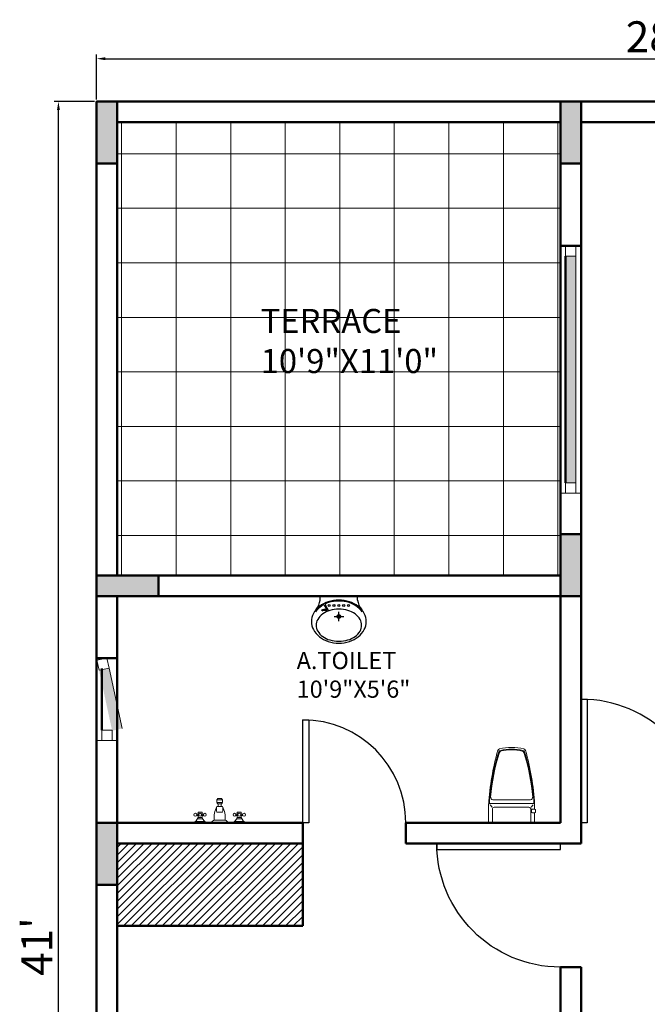
# Model space of a CAD drawing. Units: inches. Extents: x 3064 to 19385, y 846 to 15425.
# Tile 18 of 108: x 3625 to 3808, y 1134 to 1420. Entities that reach past the tile are written whole.
import ezdxf

# ---------------------------------------------------------------- set-up
doc = ezdxf.new("R2010")
doc.units = ezdxf.units.IN
for name, color, linetype, lineweight in [('A-ANNO-DIMS', 2, 'Continuous', 18), ('A-AREA-IDEN', 3, 'Continuous', 18), ('A-COLS', 1, 'Continuous', 35), ('A-DOOR', 3, 'Continuous', 25), ('A-FLOR-FIXT', 9, 'Continuous', 18), ('A-FLOR-PATT', 252, 'Continuous', 13), ('A-FURN-PATT', 252, 'Continuous', 13), ('A-GLAZ', 4, 'Continuous', 18), ('A-WALL', 7, 'Continuous', 50)]:
    doc.layers.add(name, color=color, linetype=linetype, lineweight=lineweight)
doc.layers.add('THIET-BI', color=21, linetype='Continuous')
doc.styles.get("Standard").update_dxf_attribs({"font": 'arial.ttf'})
doc.dimstyles.new('ISO-25', dxfattribs={"dimtxt": 9, "dimasz": 2.5, "dimexe": 1.25, "dimexo": 0.625, "dimtad": 1, "dimdec": 1, "dimlunit": 3, "dimtxsty": 'Standard', "dimcen": 2.5, "dimadec": 0, "dimazin": 0, "dimtfac": 1, "dimtdec": 1, "dimtmove": 0, "dimatfit": 3, "dimfxl": 1, "dimarcsym": 0})

# ---------------------------------------------------------------- blocks, each defined once
blk = doc.blocks.new('*U3')
for p, q in [((0, 0), (0, -6)), ((36, 0), (36, -6))]:
    blk.add_line(p, q)
blk.add_lwpolyline([(0, 0), (0, 36), (1.75, 36), (1.75, 0)], close=True)
blk.add_arc((0, 0), 36, 0, 90)
blk = doc.blocks.new('*U4')
for p, q in [((0, 0), (0, -6)), ((30, 0), (30, -6))]:
    blk.add_line(p, q)
blk.add_lwpolyline([(0, 0), (0, 30), (1.75, 30), (1.75, 0)], close=True)
blk.add_arc((0, 0), 30, 0, 90)
blk = doc.blocks.new('A$C430D11A0')
at = {"layer": 'THIET-BI'}
for p, q in [((90, 445), (90, 485)), ((475, 485), (90, 485)), ((475, 483), (90, 483)), ((475, 445), (475, 485)), ((129, 398), (158, 344)), ((138, 403), (176, 332)), ((282, 226), (282, 325)), ((233, 275), (332, 275))]:
    blk.add_line(p, q, dxfattribs=at)
for points in [[(565, 223, 0.121635), (545, 305, 0.10526), (482, 380, 0.088175), (393, 427, 0.079002), (282, 445, 0.079002), (172, 427, 0.088175), (83, 380, 0.10526), (20, 305, 0.121635), (0, 223, 0.121635), (20, 140, 0.10526), (83, 65, 0.088175), (172, 18, 0.079002), (282, 0, 0.079002), (393, 18, 0.088175), (482, 65, 0.10526), (545, 140, 0.121635)], [(517, 185, 0.134042), (501, 245, 0.106817), (449, 302, 0.082468), (376, 337, 0.070874), (282, 350, 0.070874), (189, 337, 0.082468), (116, 302, 0.106817), (64, 245, 0.134042), (47, 185, 0.134042), (64, 125, 0.106817), (116, 68, 0.082468), (189, 33, 0.070874), (282, 20, 0.070874), (376, 33, 0.082468), (449, 68, 0.106817), (501, 125, 0.134042)]]:
    blk.add_lwpolyline(points, format="xyb", close=True, dxfattribs=at)
for points in [[(523, 322, 0.07708), (476, 372, 0.088175), (390, 418, 0.079002), (282, 435, 0.079002), (175, 418, 0.035427), (138, 403, 0.07708)], [(129, 398, 0.043566), (89, 372, 0.07708), (42, 322, 0.041486)]]:
    blk.add_lwpolyline(points, format="xyb", dxfattribs=at)
for centre, radius in [((182, 388), 10.5), ((232, 388), 10.5), ((282, 388), 10.5), ((332, 388), 10.5), ((382, 388), 10.5), ((282, 275), 20), ((282, 275), 15)]:
    blk.add_circle(centre, radius, dxfattribs=at)
for centre, radius, start, end in [((-104, 469), 195, 320.8253, 352.9557), ((669, 469), 195, 187.0443, 219.1747), ((136, 285), 62.9, 69.643, 123.4774), ((136, 285), 52.9, 55.2455, 123.4774)]:
    blk.add_arc(centre, radius, start, end, dxfattribs=at)
blk = doc.blocks.new('WC-P05')
for p, q in [((-202, 532), (-202, 439)), ((-192, 542), (263, 542)), ((-163, 542), (-163, 401)), ((234, 542), (234, 401)), ((273, 532), (273, 352)), ((-210, 430), (-210, 409)), ((-201, 439), (-180, 439)), ((-171, 430), (-171, 409)), ((-202, 400), (-202, 352)), ((-201, 400), (-180, 400)), ((-192, 342), (263, 342)), ((-167, 379), (-188, 357)), ((-143, 381), (214, 381)), ((237, 379), (258, 357)), ((-159, 303), (229, 303))]:
    blk.add_line(p, q)
blk.add_lwpolyline([(-91, -222, 0.114547), (161, -222, 0.114547)], format="xyb")
for centre, radius, start, end in [((-192, 532), 10, 90, 180), ((263, 532), 10, 0, 90), ((-201, 430), 9, 90, 180), ((-201, 409), 9, 180, 270), ((-180, 430), 9, 0, 90), ((-180, 409), 9, 270, 0), ((2309, 492), 2515, 183.2067, 196.1242), ((-192, 352), 10, 180, 270), ((1906, 447), 2103, 182.8743, 197.6554), ((-143, 401), 20, 180, 270), ((-1836, 447), 2103, 342.3446, 357.1257), ((-2239, 492), 2515, 343.8727, 356.7933), ((214, 401), 20, 270, 0), ((263, 352), 10, 270, 0), ((-159, 280), 22.5, 90, 184.6246), ((1906, 447), 2095, 184.6245, 197.5277), ((-1836, 447), 2095, 342.464, 355.3754), ((229, 280), 22.5, 355.3754, 90), ((-76, -184), 22.5, 197.6554, 257.5059), ((-70, -177), 22.5, 197.5277, 258.1005), ((36, 324), 535, 258.1005, 281.7373), ((140, -177), 22.5, 281.7373, 342.464), ((146, -184), 22.5, 282.4941, 342.3446), ((-86, -200), 22.5, 196.1242, 256.8994), ((35, 318), 536, 257.5059, 282.4941), ((156, -200), 22.5, 283.0378, 343.8727)]:
    blk.add_arc(centre, radius, start, end)
blk = doc.blocks.new('Faucet - Bathroom front')
for p, q in [((-0.5, 4.25), (0.5, 4.25)), ((0.5, 3.75), (-0.5, 3.75)), ((-0.5, 3), (0.5, 3)), ((0.5, 2), (-0.5, 2)), ((-0.25, 3), (-0.25, 3.5)), ((0.25, 3.5), (0.25, 3)), ((-5, 0), (-2.25, 0)), ((-4.5087, 0.25), (-2.7408, 0.25)), ((-4, 1.625), (-4.25, 1.625)), ((-4, 1.375), (-4.25, 1.375)), ((-3.1442, 0.75), (-4.0979, 0.75)), ((-3.25, 1.625), (-3, 1.625)), ((-3.25, 1.375), (-3, 1.375)), ((-1.5, 0), (1.5, 0)), ((-1, 0.5), (1, 0.5)), ((2.25, 0), (5, 0)), ((2.7413, 0.25), (4.5092, 0.25)), ((3.25, 1.625), (3, 1.625)), ((3.25, 1.375), (3, 1.375)), ((4.1058, 0.75), (3.1521, 0.75)), ((4, 1.625), (4.25, 1.625)), ((4, 1.375), (4.25, 1.375))]:
    blk.add_line(p, q)
for points in [[(-0.5, 3.75), (-0.5, 4.25)], [(-0.25, 4.5), (0.25, 4.5)], [(0.5, 4.25), (0.5, 3.75)], [(0.25, 3.5), (-0.25, 3.5)]]:
    blk.add_lwpolyline(points)
for points in [[(-4, 1), (-4, 2), (-3.25, 2), (-3.25, 1)], [(3.25, 1), (3.25, 2), (4, 2), (4, 1)]]:
    blk.add_lwpolyline(points, close=True)
for centre in [(-4.5, 1.5), (-3.625, 1.5), (-2.75, 1.5), (2.75, 1.5), (3.625, 1.5), (4.5, 1.5)]:
    blk.add_circle(centre, 0.2795)
for centre, radius, start, end in [((-0.2575, 4.2575), 0.2426, 88.22243, 181.7776), ((-0.2575, 3.7425), 0.2426, 178.2224, 271.7776), ((0.2575, 4.2575), 0.2426, 358.2224, 91.77757), ((0.2575, 3.7425), 0.2426, 268.2224, 1.777565), ((3, 1), 4.0311, 150.2551, 187.125), ((0.6413, 2.5), 1.246, 156.3417, 203.6583), ((-3, 1), 4.0311, 352.875, 29.74488), ((-0.6413, 2.5), 1.246, 336.3417, 23.65835), ((-5.375, 1.375), 1.4252, 285.2551, 344.7449), ((-1.875, 1.375), 1.4252, 195.2551, 254.7449), ((-0.7962, -0.2038), 0.7327, 106.1502, 163.8498), ((0.7962, -0.2038), 0.7327, 16.1502, 73.84979), ((1.875, 1.375), 1.4252, 285.2551, 344.7449), ((5.375, 1.375), 1.4252, 195.2551, 254.7449)]:
    blk.add_arc(centre, radius, start, end)
blk = doc.blocks.new('*D40')
at = {"layer": 'A-ANNO-DIMS', "color": 0, "lineweight": -2, "transparency": 16777216}
for p, q in [((3646.73, 1396.34), (3634.99, 1396.34)), ((3636.24, 906.84), (3636.24, 1393.84)), ((3646.73, 904.34), (3634.99, 904.34))]:
    blk.add_line(p, q, dxfattribs=at)
at = {"layer": 'A-ANNO-DIMS', "color": 0, "transparency": 16777216}
for points in [[(3635.82, 1393.84), (3636.66, 1393.84), (3636.24, 1396.34)], [(3635.82, 906.84), (3636.66, 906.84), (3636.24, 904.34)]]:
    blk.add_solid(points, dxfattribs=at)
at = {"layer": 'Defpoints', "color": 0, "transparency": 16777216}
for p in [(3636.24, 1396.34), (3647.36, 1396.34), (3647.36, 904.34)]:
    blk.add_point(p, dxfattribs=at)
at = {"layer": 'A-ANNO-DIMS', "color": 0, "transparency": 16777216, "insert": (3631.1, 1150.34), "char_height": 9, "attachment_point": 5, "rotation": 90}
blk.add_mtext("41'", dxfattribs=at)
blk = doc.blocks.new('*D41')
at = {"layer": 'A-ANNO-DIMS', "color": 0, "lineweight": -2, "transparency": 16777216}
for p, q in [((3647.36, 1396.96), (3647.36, 1410.06)), ((3649.86, 1408.81), (3986.86, 1408.81)), ((3989.36, 1396.96), (3989.36, 1410.06))]:
    blk.add_line(p, q, dxfattribs=at)
at = {"layer": 'A-ANNO-DIMS', "color": 0, "transparency": 16777216}
for points in [[(3649.86, 1409.23), (3649.86, 1408.39), (3647.36, 1408.81)], [(3986.86, 1409.23), (3986.86, 1408.39), (3989.36, 1408.81)]]:
    blk.add_solid(points, dxfattribs=at)
at = {"layer": 'Defpoints', "color": 0, "transparency": 16777216}
for p in [(3989.36, 1408.81), (3647.36, 1396.34), (3989.36, 1396.34)]:
    blk.add_point(p, dxfattribs=at)
at = {"layer": 'A-ANNO-DIMS', "color": 0, "transparency": 16777216, "insert": (3818.36, 1414.03), "char_height": 9, "attachment_point": 5}
blk.add_mtext('28\'-6"', dxfattribs=at)
blk = doc.blocks.new('WIN-600')
h = blk.add_hatch(color=256)
h.dxf.hatch_style = 1
h.paths.add_polyline_path([(3, 18), (0, 18), (0, 0), (3, 0)])
blk.add_line((3, 18), (3, 0))
blk.add_lwpolyline([(3, 18), (0, 18), (0, 21), (3, 21)], close=True)
blk = doc.blocks.new('WIN-1900')
blk.add_line((3, 0), (3, 66))
blk.add_lwpolyline([(3, 66), (0, 66), (0, 69), (3, 69)], close=True)

msp = doc.modelspace()

# ---------------------------------------------------------------- hatches: boundary and pattern name
at = {"layer": 'A-COLS'}
h = msp.add_hatch(color=256, dxfattribs=at)
h.dxf.hatch_style = 1
h.paths.add_polyline_path([(3647.36, 1378.34), (3653.36, 1378.34), (3653.36, 1396.34), (3647.36, 1396.34)])
h = msp.add_hatch(color=256, dxfattribs=at)
h.dxf.hatch_style = 1
h.paths.add_polyline_path([(3782.36, 1378.34), (3788.36, 1378.34), (3788.36, 1396.34), (3782.36, 1396.34)])
h = msp.add_hatch(color=256, dxfattribs=at)
h.dxf.hatch_style = 1
h.paths.add_polyline_path([(3782.36, 1252.34), (3788.36, 1252.34), (3788.36, 1270.34), (3782.36, 1270.34)])
h = msp.add_hatch(color=256, dxfattribs=at)
h.dxf.hatch_style = 1
h.paths.add_polyline_path([(3665.36, 1252.34), (3665.36, 1258.34), (3647.36, 1258.34), (3647.36, 1252.34)])
h = msp.add_hatch(color=256, dxfattribs=at)
h.dxf.hatch_style = 1
h.paths.add_polyline_path([(3647.36, 1168.34), (3653.36, 1168.34), (3653.36, 1186.34), (3647.36, 1186.34)])
at = {"layer": 'A-FLOR-PATT'}
h = msp.add_hatch(dxfattribs=at)
h.set_pattern_fill('ANSI37', color=256, scale=5, angle=45)
h.set_pattern_definition([(90, (-695.134, 0), (-15.875, 0), []), (180, (-695.134, 0), (-2e-15, -15.875), [])])
h.paths.add_polyline_path([(3653.36, 1390.34), (3653.36, 1378.34), (3653.36, 1258.34), (3782.36, 1258.34), (3782.36, 1270.34), (3782.36, 1390.34)])
at = {"layer": 'A-FURN-PATT'}
h = msp.add_hatch(dxfattribs=at)
h.set_pattern_fill('ANSI31', color=256, scale=0.5)
h.set_pattern_definition([(45, (-695.1336, -6), (-1.122532, 1.122532), [])])
h.paths.add_polyline_path([(3707.36, 1180.34), (3653.36, 1180.34), (3653.36, 1162.34), (3653.36, 1156.34), (3707.36, 1156.34)])
at = {"layer": 'A-GLAZ'}
h = msp.add_hatch(color=256, dxfattribs=at)
h.dxf.hatch_style = 1
h.paths.add_polyline_path([(3783.86, 1285.34), (3786.86, 1285.34), (3786.86, 1351.34), (3783.86, 1351.34)])

# ---------------------------------------------------------------- linework, layer by layer
for p, q in [((3788.36, 1282.34), (3782.36, 1282.34)), ((3647.36, 1210.28), (3653.36, 1210.28))]:
    msp.add_line(p, q, dxfattribs=at)
for points in [[(3786.86, 1282.34), (3783.86, 1282.34), (3783.86, 1285.34), (3786.86, 1285.34)], [(3651.86, 1210.28), (3648.86, 1210.28), (3648.86, 1213.28), (3651.86, 1213.28)]]:
    msp.add_lwpolyline(points, close=True, dxfattribs=at)
at = {"layer": 'A-WALL'}
for p, q in [((3989.36, 1396.34), (3647.36, 1396.34)), ((3647.36, 1396.34), (3647.36, 976.34)), ((3782.36, 1390.34), (3653.36, 1390.34)), ((3653.36, 1390.34), (3653.36, 1258.34)), ((3782.36, 1390.34), (3782.36, 1258.34)), ((3983.36, 1390.34), (3788.36, 1390.34)), ((3788.36, 1390.34), (3788.36, 1180.34)), ((3782.36, 1354.34), (3788.36, 1354.34)), ((3783.86, 1351.34), (3783.86, 1285.34)), ((3653.36, 1258.34), (3782.36, 1258.34)), ((3653.36, 1252.34), (3782.36, 1252.34)), ((3653.36, 1252.34), (3653.36, 1186.34)), ((3788.36, 1252.34), (3782.36, 1252.34)), ((3782.36, 1252.34), (3782.36, 1186.34)), ((3647.36, 1234.28), (3653.36, 1234.28)), ((3648.86, 1231.28), (3648.86, 1213.28)), ((3653.36, 1186.34), (3707.36, 1186.34)), ((3707.36, 1186.34), (3707.36, 1156.34)), ((3737.36, 1186.34), (3737.36, 1180.34)), ((3737.36, 1186.34), (3782.36, 1186.34)), ((3653.36, 1180.34), (3707.36, 1180.34)), ((3653.36, 1180.34), (3653.36, 982.34)), ((3737.36, 1180.34), (3788.36, 1180.34)), ((3653.36, 1156.34), (3707.36, 1156.34)), ((3782.36, 1144.34), (3788.36, 1144.34)), ((3782.36, 1144.34), (3782.36, 982.34)), ((3788.36, 1144.34), (3788.36, 976.34))]:
    msp.add_line(p, q, dxfattribs=at)
for points in [[(3653.36, 1378.34), (3653.36, 1396.34), (3647.36, 1396.34), (3647.36, 1378.34)], [(3788.36, 1378.34), (3788.36, 1396.34), (3782.36, 1396.34), (3782.36, 1378.34)], [(3788.36, 1252.34), (3788.36, 1270.34), (3782.36, 1270.34), (3782.36, 1252.34)], [(3665.36, 1258.34), (3647.36, 1258.34), (3647.36, 1252.34), (3665.36, 1252.34)], [(3653.36, 1168.34), (3653.36, 1186.34), (3647.36, 1186.34), (3647.36, 1168.34)]]:
    msp.add_lwpolyline(points, close=True, dxfattribs=at)

# ---------------------------------------------------------------- block references
at = {"layer": 'A-DOOR'}
for name, p in [('*U3', (3788.36, 1186.34)), ('*U4', (3707.36, 1186.34))]:
    msp.add_blockref(name, p, dxfattribs=at)
at = {"layer": 'A-DOOR', "xscale": -1, "rotation": 90}
msp.add_blockref('*U3', (3782.36, 1180.34), dxfattribs=at)
at = {"layer": 'A-FLOR-FIXT'}
for name, p, xscale, yscale, zscale in [('A$C430D11A0', (3709.89, 1238.65), 0.0282220760332506, 0.0282220760332506, 0.0282220760332506), ('Faucet - Bathroom front', (3683.17, 1186.34), 1.573166238287219, 1.573166238287219, 1.573166238287219)]:
    msp.add_blockref(name, p, dxfattribs=dict(at, xscale=xscale, yscale=yscale, zscale=zscale))
at = {"layer": 'A-FLOR-FIXT', "xscale": 0.0282220760332506, "yscale": 0.0282220760332506, "zscale": 0.0282220760332506, "rotation": 180}
msp.add_blockref('WC-P05', (3769.14, 1201.63), dxfattribs=at)
at = {"layer": 'A-GLAZ'}
msp.add_blockref('WIN-1900', (3783.86, 1285.34), dxfattribs=at)
at = {"layer": 'A-GLAZ', "rotation": 12.21571913412907}
msp.add_blockref('WIN-600', (3651.87, 1213.17), dxfattribs=at)

# ---------------------------------------------------------------- texts
at = {"layer": 'A-AREA-IDEN', "attachment_point": 1}
for s, insert, char_height in [('TERRACE\\P10\'9"X11\'0"', (3695.09, 1335.96), 7), ('A.TOILET\\P10\'9"X5\'6"', (3705.58, 1236.1), 5)]:
    msp.add_mtext_dynamic_manual_height_columns(s, width=67.5924, gutter_width=12.5, heights=[0], dxfattribs=dict(at, insert=insert, char_height=char_height))

# ---------------------------------------------------------------- dimensions: what is measured, and where the dimension line sits
at = {"layer": 'A-ANNO-DIMS'}
dim = msp.add_linear_dim(base=(3989.36, 1408.81), p1=(3647.36, 1396.34), p2=(3989.36, 1396.34), dimstyle='ISO-25', override={"dimclrd": 0, "dimclre": 0, "dimclrt": 0}, dxfattribs=at)
dim.commit()
dim.dimension.update_dxf_attribs({"geometry": '*D41', "text_midpoint": (3818.36, 1414.03)})
dim = msp.add_linear_dim(base=(3636.24, 1396.34), p1=(3647.36, 904.34), p2=(3647.36, 1396.34), angle=90, dimstyle='ISO-25', override={"dimclrd": 0, "dimclre": 0, "dimclrt": 0}, dxfattribs=at)
dim.commit()
dim.dimension.update_dxf_attribs({"geometry": '*D40', "text_midpoint": (3631.1, 1150.34)})

doc.saveas('drawing.dxf')
